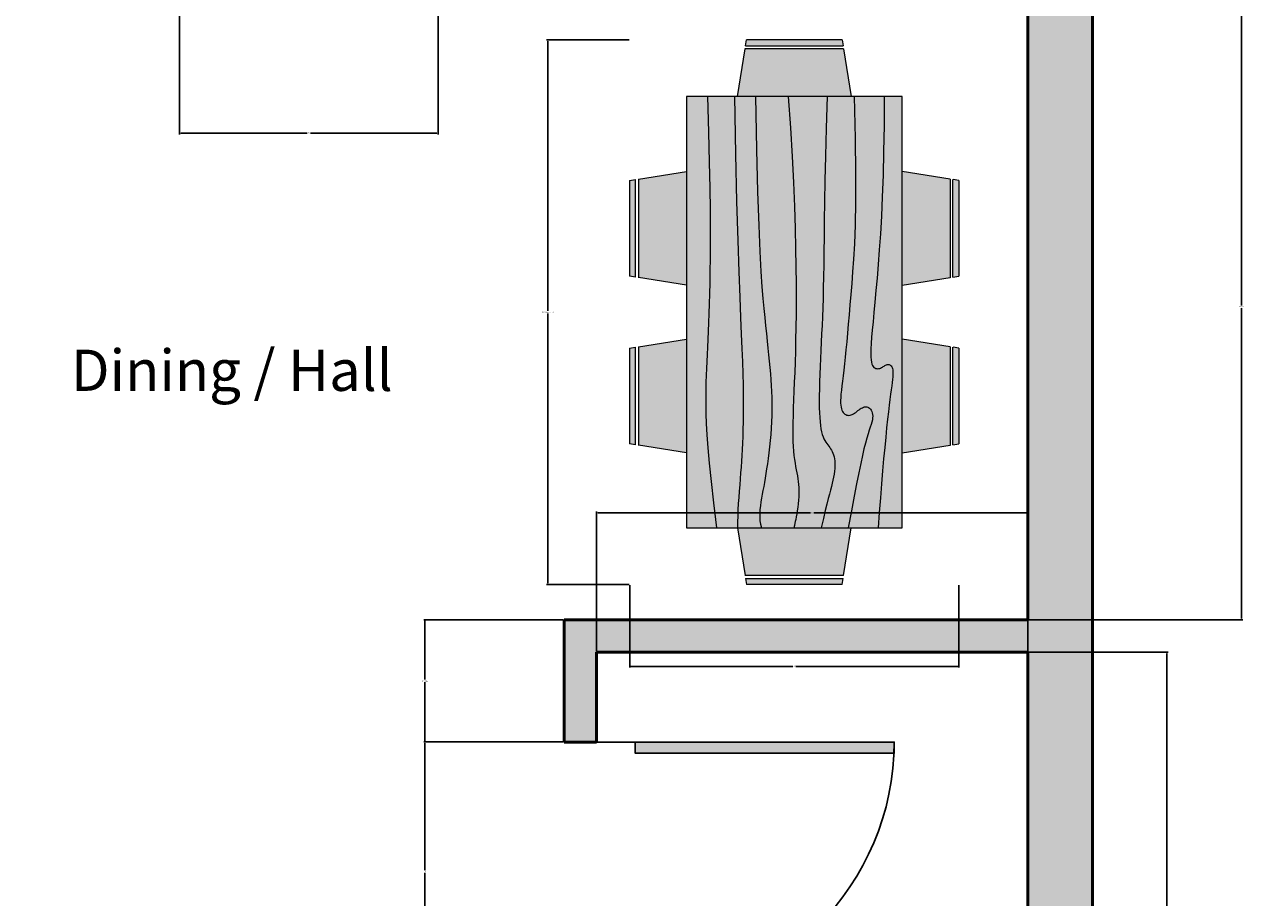
# Model space of a CAD drawing. Units: inches. Extents: x 2578 to 2919, y 51 to 451.
# Tile 4 of 5: x 2750 to 2919, y 172 to 293. Entities that reach past the tile are written whole.
import ezdxf

# ---------------------------------------------------------------- set-up
doc = ezdxf.new("R2010")
doc.units = ezdxf.units.IN
for name, color, linetype, lineweight in [('A-ANNO-DIMS', 2, 'Continuous', 18), ('A-AREA-IDEN', 7, 'Continuous', 25), ('A-DOOR', 4, 'Continuous', 25), ('A-FURN', 8, 'Continuous', 18), ('A-FURN-PATT', 253, 'Continuous', 13), ('A-WALL', 7, 'Continuous', 50), ('A-WALL-PATT', 250, 'Continuous', 13)]:
    doc.layers.add(name, color=color, linetype=linetype, lineweight=lineweight)
doc.layers.add('A-DOOR-PATT', color=29, linetype='Continuous', lineweight=13, true_color=0x4f342a)
doc.styles.get("Standard").update_dxf_attribs({"font": 'arial.ttf'})
doc.dimstyles.get("Standard").update_dxf_attribs({"dimtxt": 0.18, "dimasz": 0.18, "dimexe": 0.18, "dimexo": 0.0625, "dimgap": 0.09, "dimtad": 0, "dimtih": 1, "dimtoh": 1, "dimdec": 4, "dimzin": 0, "dimdsep": 46, "dimtxsty": 'Standard', "dimcen": 0.09, "dimadec": 0, "dimazin": 0, "dimtfac": 1, "dimtdec": 4, "dimtofl": 0, "dimtmove": 0, "dimatfit": 3, "dimfxl": 1, "dimtolj": 1, "dimtzin": 0, "dimarcsym": 0})

# ---------------------------------------------------------------- blocks, each defined once
blk = doc.blocks.new('*U3')
for p, q in [((0, 0), (0, -6)), ((40, 0), (40, -6))]:
    blk.add_line(p, q)
blk.add_lwpolyline([(0, 0), (0, 40), (1.75, 40), (1.75, 0)], close=True)
blk.add_arc((0, 0), 40, 0, 90)
blk = doc.blocks.new('Dining Set - 36 x 72 in.')
for p, q in [((-22, 27.5), (-22.1562, 26.50042)), ((-5.8416, 26.5), (-22.1534, 26.5)), ((-22, 27.5), (-6, 27.5)), ((-5.8437, 26.49966), (-6, 27.5)), ((6, 27.5), (5.8438, 26.50042)), ((22.1584, 26.5), (5.8466, 26.5)), ((6, 27.5), (22, 27.5)), ((22.1563, 26.49966), (22, 27.5)), ((-22.2343, 26.00059), (-23.4847, 17.99762)), ((-22.2304, 26), (-5.7608, 26)), ((-4.5152, 17.99762), (-5.7655, 25.99926)), ((5.7657, 26.00059), (4.5153, 17.99762)), ((5.7696, 26), (22.2392, 26)), ((23.4848, 17.99762), (22.2345, 25.99926)), ((36, 18), (-36, 18)), ((-36, 18), (-36, -18)), ((36, -18), (36, 18)), ((-45.5, 8), (-44.5004, 8.15617)), ((-44.5, -8.15843), (-44.5, 8.15338)), ((-44.0006, 8.23428), (-35.9976, 9.48474)), ((-44, 8.23041), (-44, -8.23915)), ((44.0006, 8.23428), (35.9976, 9.48474)), ((44, 8.23041), (44, -8.23915)), ((44.5, -8.15843), (44.5, 8.15338)), ((45.5, 8), (44.5005, 8.15617)), ((-45.5, 8), (-45.5, -8)), ((45.5, 8), (45.5, -8)), ((-44.4997, -8.15631), (-45.5, -8)), ((44.4997, -8.15631), (45.5, -8)), ((-35.9976, -9.48476), (-43.9993, -8.2345)), ((35.9976, -9.48476), (43.9993, -8.2345)), ((-36, -18), (36, -18)), ((-22.2343, -26.0006), (-23.4847, -17.99762)), ((-4.5152, -17.99762), (-5.7655, -25.99928)), ((5.7657, -26.0006), (4.5153, -17.99762)), ((23.4848, -17.99762), (22.2345, -25.99928)), ((-22.2304, -26), (-5.7608, -26)), ((5.7696, -26), (22.2392, -26)), ((-22, -27.5), (-22.1562, -26.50044)), ((-5.8416, -26.5), (-22.1534, -26.5)), ((-22, -27.5), (-6, -27.5)), ((-5.8437, -26.49967), (-6, -27.5)), ((6, -27.5), (5.8438, -26.50044)), ((22.1584, -26.5), (5.8466, -26.5)), ((6, -27.5), (22, -27.5)), ((22.1563, -26.49967), (22, -27.5))]:
    blk.add_line(p, q)
for points in [[(-36, 15), (-31.1772, 14.97754), (-26.8079, 14.91406), (-22.8538, 14.81543), (-19.276, 14.6875), (-16.0362, 14.53613), (-13.0957, 14.36718), (-10.4159, 14.18652), (-7.9583, 14), (-5.6904, 13.81315), (-3.6035, 13.63021), (-1.6954, 13.45508), (0.0365, 13.29166), (1.5945, 13.14388), (2.9811, 13.01562), (4.1988, 12.9108), (5.25, 12.83333), (6.1393, 12.78613), (6.8802, 12.76823), (7.4883, 12.77767), (7.9792, 12.8125), (8.3685, 12.87077), (8.6719, 12.95052), (8.9049, 13.0498), (9.0833, 13.16666), (9.2205, 13.29899), (9.3216, 13.44401), (9.3895, 13.59879), (9.4271, 13.76041), (9.4373, 13.92594), (9.4232, 14.09245), (9.3875, 14.257), (9.3333, 14.41666), (9.2638, 14.56917), (9.1836, 14.71484), (9.0975, 14.85465), (9.0104, 14.98958), (8.9272, 15.1206), (8.8529, 15.2487), (8.7922, 15.37483), (8.75, 15.5), (8.7305, 15.62467), (8.7344, 15.74739), (8.7617, 15.86621), (8.8125, 15.97916), (8.8867, 16.08431), (8.9844, 16.17968), (9.1055, 16.26334), (9.25, 16.33333), (9.4189, 16.38802), (9.6172, 16.42708), (9.8506, 16.45052), (10.125, 16.45833), (10.4463, 16.45052), (10.8203, 16.42708), (11.2529, 16.38802), (11.75, 16.33333), (12.3184, 16.26318), (12.9694, 16.17838), (13.7151, 16.07991), (14.5677, 15.96875), (15.5395, 15.84586), (16.6426, 15.71224), (17.8893, 15.56884), (19.2917, 15.41666), (20.859, 15.25667), (22.5879, 15.08984), (24.4721, 14.91715), (26.5052, 14.73958), (28.6809, 14.5581), (30.9929, 14.3737), (33.4347, 14.18733), (36, 14)], [(-36, 10), (-28.9766, 10.14274), (-23.1725, 10.20442), (-18.4241, 10.19775), (-14.5677, 10.13541), (-11.4399, 10.03011), (-8.877, 9.89453), (-6.7154, 9.74137), (-4.7917, 9.58333), (-2.9698, 9.43082), (-1.2246, 9.28515), (0.4415, 9.14534), (2.026, 9.01041), (3.5266, 8.87939), (4.9408, 8.7513), (6.266, 8.62516), (7.5, 8.5), (8.6411, 8.37549), (9.6914, 8.2539), (10.6538, 8.13818), (11.5312, 8.03125), (12.3267, 7.93603), (13.043, 7.85547), (13.6831, 7.79248), (14.25, 7.75), (14.7471, 7.7303), (15.1797, 7.73307), (15.5537, 7.75732), (15.875, 7.80208), (16.1494, 7.86637), (16.3828, 7.94922), (16.5811, 8.04964), (16.75, 8.16666), (16.8944, 8.29915), (17.0143, 8.44531), (17.1089, 8.60319), (17.1771, 8.77083), (17.218, 8.94629), (17.2305, 9.1276), (17.2137, 9.31282), (17.1667, 9.5), (17.0895, 9.6875), (16.987, 9.875), (16.8649, 10.0625), (16.7292, 10.25), (16.5856, 10.4375), (16.4401, 10.625), (16.2985, 10.8125), (16.1667, 11), (16.05, 11.18733), (15.9518, 11.3737), (15.8752, 11.5581), (15.8229, 11.73958), (15.798, 11.91715), (15.8034, 12.08984), (15.842, 12.25667), (15.9167, 12.41666), (16.0295, 12.56836), (16.1784, 12.70833), (16.3605, 12.83268), (16.5729, 12.9375), (16.8127, 13.01888), (17.0768, 13.07291), (17.3625, 13.0957), (17.6667, 13.08333), (17.9894, 13.03312), (18.3418, 12.94726), (18.7382, 12.82918), (19.1927, 12.68229), (19.7195, 12.51001), (20.3327, 12.31575), (21.0465, 12.10294), (21.875, 11.875), (22.8357, 11.63354), (23.959, 11.37304), (25.2786, 11.08618), (26.8282, 10.76562), (28.6414, 10.40405), (30.752, 9.99414), (33.1936, 9.52856), (36, 9)], [(-36, 5.5), (-30.7157, 5.3348), (-26.069, 5.20963), (-21.9946, 5.11767), (-18.4271, 5.05208), (-15.3009, 5.00602), (-12.5508, 4.97265), (-10.1112, 4.94515), (-7.9167, 4.91666), (-5.909, 4.88167), (-4.0586, 4.83984), (-2.3429, 4.79215), (-0.7396, 4.73958), (0.7739, 4.6831), (2.22, 4.6237), (3.6213, 4.56233), (5, 4.5), (6.373, 4.43782), (7.7344, 4.3776), (9.0723, 4.32129), (10.375, 4.27083), (11.6309, 4.22819), (12.8281, 4.19531), (13.9551, 4.17415), (15, 4.16666), (15.954, 4.17448), (16.819, 4.19791), (17.6001, 4.23698), (18.3021, 4.29166), (18.9299, 4.36198), (19.4883, 4.44791), (19.9823, 4.54948), (20.4167, 4.66666), (20.7969, 4.79899), (21.1302, 4.94401), (21.4245, 5.09879), (21.6875, 5.26041), (21.9271, 5.42594), (22.1511, 5.59245), (22.3672, 5.757), (22.5834, 5.91666), (22.8065, 6.06868), (23.0404, 6.21093), (23.2879, 6.34147), (23.5521, 6.45833), (23.8358, 6.55957), (24.142, 6.64323), (24.4735, 6.70735), (24.8334, 6.75), (25.2235, 6.76969), (25.642, 6.76692), (26.0858, 6.74267), (26.5521, 6.69791), (27.0379, 6.63362), (27.5404, 6.55078), (28.0565, 6.45036), (28.5834, 6.33333), (29.1242, 6.19987), (29.7071, 6.04687), (30.3661, 5.87044), (31.1354, 5.66666), (32.0493, 5.43164), (33.142, 5.16146), (34.4475, 4.85221), (36, 4.5)], [(-36, -1), (-30.7915, -0.6591), (-26.0195, -0.38216), (-21.6519, -0.16284), (-17.6563, 0.00521), (-14.0005, 0.12833), (-10.6523, 0.21289), (-7.5796, 0.26522), (-4.75, 0.29166), (-2.134, 0.29793), (0.2878, 0.28711), (2.5317, 0.26163), (4.6146, 0.22396), (6.5529, 0.17651), (8.3633, 0.12174), (10.0623, 0.06209), (11.6667, 0), (13.1899, -0.06201), (14.6341, -0.1211), (15.9982, -0.17432), (17.2813, -0.21875), (18.4823, -0.25147), (19.6003, -0.26953), (20.6343, -0.27002), (21.5834, -0.25), (22.4481, -0.20768), (23.2357, -0.14584), (23.9549, -0.06836), (24.6146, 0.02083), (25.2235, 0.11784), (25.7904, 0.21875), (26.3241, 0.31966), (26.8334, 0.41666), (27.3265, 0.50618), (27.8099, 0.58593), (28.2894, 0.65397), (28.7709, 0.70833), (29.2601, 0.74707), (29.763, 0.76823), (30.2855, 0.76985), (30.8334, 0.75), (31.4088, 0.70784), (31.9994, 0.64713), (32.589, 0.57275), (33.1615, 0.48958), (33.7008, 0.4025), (34.1908, 0.3164), (34.6153, 0.23616), (34.9584, 0.16666), (35.2099, 0.11165), (35.3848, 0.07031), (35.504, 0.04069), (35.5886, 0.02083), (35.6594, 0.00879), (35.7377, 0.0026), (35.8442, 0.00032), (36, 0)], [(-36, -6.5), (-27.1843, -6.31267), (-20.084, -6.1263), (-14.469, -5.9419), (-10.1094, -5.76042), (-6.7752, -5.58285), (-4.2363, -5.41016), (-2.2629, -5.24333), (-0.625, -5.08334), (0.8708, -4.93099), (2.2715, -4.78646), (3.5872, -4.64974), (4.8281, -4.52084), (6.0046, -4.39974), (7.127, -4.28646), (8.2053, -4.18099), (9.25, -4.08334), (10.2705, -3.99382), (11.2734, -3.91407), (12.2647, -3.84603), (13.25, -3.79167), (14.2354, -3.75293), (15.2266, -3.73177), (16.2295, -3.73015), (17.25, -3.75), (18.2912, -3.79248), (19.3451, -3.85547), (20.4009, -3.93604), (21.4479, -4.03125), (22.4754, -4.13819), (23.4727, -4.25391), (24.4289, -4.37549), (25.3334, -4.5), (26.1785, -4.62492), (26.9694, -4.74935), (27.7145, -4.87281), (28.4219, -4.99479), (29.1, -5.11483), (29.7572, -5.23242), (30.4016, -5.34709), (31.0417, -5.45834), (31.6837, -5.56437), (32.3262, -5.65821), (32.9658, -5.73153), (33.599, -5.77604), (34.2224, -5.78345), (34.8327, -5.74545), (35.4264, -5.65373), (36, -5.5)], [(-36, -10), (-26.4022, -9.81299), (-18.4675, -9.62891), (-11.9839, -9.45069), (-6.7396, -9.28125), (-2.5226, -9.12354), (0.8789, -8.98047), (3.6769, -8.85498), (6.0833, -8.75), (8.2767, -8.66765), (10.3021, -8.60677), (12.1712, -8.56543), (13.8958, -8.54167), (15.4876, -8.53353), (16.9583, -8.53907), (18.3197, -8.55632), (19.5834, -8.58334), (20.7616, -8.61841), (21.8685, -8.66081), (22.9188, -8.71004), (23.9271, -8.76563), (24.9081, -8.82707), (25.8763, -8.89388), (26.8465, -8.96558), (27.8334, -9.04167), (28.8474, -9.12118), (29.8828, -9.20117), (30.93, -9.27824), (31.9792, -9.34896), (33.0205, -9.40991), (34.0443, -9.45768), (35.0407, -9.48885), (36, -9.5)], [(-36, -14.5), (-30.0881, -14.33513), (-25.0332, -14.21224), (-20.7312, -14.12647), (-17.0781, -14.07292), (-13.97, -14.04671), (-11.3027, -14.04297), (-8.9724, -14.05681), (-6.875, -14.08334), (-4.9224, -14.11833), (-3.0905, -14.16016), (-1.3709, -14.20785), (0.2448, -14.26042), (1.7647, -14.3169), (3.1973, -14.3763), (4.5507, -14.43767), (5.8333, -14.5), (7.0554, -14.5621), (8.235, -14.62175), (9.3922, -14.67652), (10.5469, -14.72396), (11.7192, -14.76164), (12.929, -14.78711), (14.1965, -14.79794), (15.5417, -14.79167), (16.9933, -14.76424), (18.6152, -14.70508), (20.4804, -14.60197), (22.6615, -14.44271), (25.2312, -14.21509), (28.2624, -13.9069), (31.8277, -13.50594), (36, -13)]]:
    blk.add_lwpolyline(points)
blk = doc.blocks.new('*D27')
at = {"layer": 'A-ANNO-DIMS', "color": 0, "lineweight": -2, "transparency": 16777216}
for p, q in [((2833.73, 291.27), (2822.25, 291.27)), ((2822.43, 291.09), (2822.43, 253.56)), ((2822.43, 215.67), (2822.43, 253.2)), ((2833.73, 215.49), (2822.25, 215.49))]:
    blk.add_line(p, q, dxfattribs=at)
at = {"layer": 'A-ANNO-DIMS', "color": 0, "transparency": 16777216}
for points in [[(2822.4, 291.09), (2822.46, 291.09), (2822.43, 291.27)], [(2822.4, 215.67), (2822.46, 215.67), (2822.43, 215.49)]]:
    blk.add_solid(points, dxfattribs=at)
at = {"layer": 'Defpoints', "color": 0, "transparency": 16777216}
for p in [(2833.8, 291.27), (2822.43, 215.49), (2833.8, 215.49)]:
    blk.add_point(p, dxfattribs=at)
at = {"layer": 'A-ANNO-DIMS', "color": 0, "transparency": 16777216, "insert": (2822.43, 253.38), "char_height": 0.18, "attachment_point": 5}
blk.add_mtext('\\A1;DINING SET 76', dxfattribs=at)
blk = doc.blocks.new('*D28')
at = {"layer": 'A-ANNO-DIMS', "color": 0, "lineweight": -2, "transparency": 16777216}
for p, q in [((2833.8, 215.43), (2833.8, 203.94)), ((2879.6, 215.43), (2879.6, 203.94)), ((2833.98, 204.12), (2856.48, 204.12)), ((2879.42, 204.12), (2856.92, 204.12))]:
    blk.add_line(p, q, dxfattribs=at)
at = {"layer": 'A-ANNO-DIMS', "color": 0, "transparency": 16777216}
for points in [[(2833.98, 204.15), (2833.98, 204.09), (2833.8, 204.12)], [(2879.42, 204.15), (2879.42, 204.09), (2879.6, 204.12)]]:
    blk.add_solid(points, dxfattribs=at)
at = {"layer": 'Defpoints', "color": 0, "transparency": 16777216}
for p in [(2833.8, 215.49), (2879.6, 215.49), (2879.6, 204.12)]:
    blk.add_point(p, dxfattribs=at)
at = {"layer": 'A-ANNO-DIMS', "color": 0, "transparency": 16777216, "insert": (2856.7, 204.12), "char_height": 0.18, "attachment_point": 5}
blk.add_mtext('\\A1;46', dxfattribs=at)
blk = doc.blocks.new('*D46')
at = {"layer": 'A-ANNO-DIMS', "color": 0, "lineweight": -2, "transparency": 16777216}
for p, q in [((2829.18, 206.17), (2829.18, 225.64)), ((2889.18, 206.17), (2889.18, 225.64)), ((2829.36, 225.46), (2858.96, 225.46)), ((2889, 225.46), (2859.4, 225.46))]:
    blk.add_line(p, q, dxfattribs=at)
at = {"layer": 'A-ANNO-DIMS', "color": 0, "transparency": 16777216}
for points in [[(2829.36, 225.49), (2829.36, 225.43), (2829.18, 225.46)], [(2889, 225.49), (2889, 225.43), (2889.18, 225.46)]]:
    blk.add_solid(points, dxfattribs=at)
at = {"layer": 'Defpoints', "color": 0, "transparency": 16777216}
for p in [(2889.18, 225.46), (2829.18, 206.11), (2889.18, 206.11)]:
    blk.add_point(p, dxfattribs=at)
at = {"layer": 'A-ANNO-DIMS', "color": 0, "transparency": 16777216, "insert": (2859.18, 225.46), "char_height": 0.18, "attachment_point": 5}
blk.add_mtext('\\A1;60', dxfattribs=at)
blk = doc.blocks.new('*D47')
at = {"layer": 'A-ANNO-DIMS', "color": 0, "lineweight": -2, "transparency": 16777216}
for p, q in [((2889.24, 206.11), (2908.71, 206.11)), ((2908.53, 205.93), (2908.53, 153.04)), ((2908.53, 99.78), (2908.53, 152.67)), ((2889.24, 99.6), (2908.71, 99.6))]:
    blk.add_line(p, q, dxfattribs=at)
at = {"layer": 'A-ANNO-DIMS', "color": 0, "transparency": 16777216}
for points in [[(2908.5, 205.93), (2908.56, 205.93), (2908.53, 206.11)], [(2908.5, 99.78), (2908.56, 99.78), (2908.53, 99.6)]]:
    blk.add_solid(points, dxfattribs=at)
at = {"layer": 'Defpoints', "color": 0, "transparency": 16777216}
for p in [(2889.18, 206.11), (2889.18, 99.6), (2908.53, 99.6)]:
    blk.add_point(p, dxfattribs=at)
at = {"layer": 'A-ANNO-DIMS', "color": 0, "transparency": 16777216, "insert": (2908.53, 152.85), "char_height": 0.18, "attachment_point": 5}
blk.add_mtext('\\A1;106.51', dxfattribs=at)
blk = doc.blocks.new('*D49')
at = {"layer": 'A-ANNO-DIMS', "color": 0, "lineweight": -2, "transparency": 16777216}
for p, q in [((2889.24, 297.64), (2919.06, 297.64)), ((2918.88, 297.46), (2918.88, 254.31)), ((2918.88, 210.79), (2918.88, 253.94)), ((2889.24, 210.61), (2919.06, 210.61))]:
    blk.add_line(p, q, dxfattribs=at)
at = {"layer": 'A-ANNO-DIMS', "color": 0, "transparency": 16777216}
for points in [[(2918.85, 297.46), (2918.91, 297.46), (2918.88, 297.64)], [(2918.85, 210.79), (2918.91, 210.79), (2918.88, 210.61)]]:
    blk.add_solid(points, dxfattribs=at)
at = {"layer": 'Defpoints', "color": 0, "transparency": 16777216}
for p in [(2889.18, 297.64), (2918.88, 297.64), (2889.18, 210.61)]:
    blk.add_point(p, dxfattribs=at)
at = {"layer": 'A-ANNO-DIMS', "color": 0, "transparency": 16777216, "insert": (2918.88, 254.13), "char_height": 0.18, "attachment_point": 5}
blk.add_mtext('\\A1;87.03', dxfattribs=at)
blk = doc.blocks.new('*D54')
at = {"layer": 'A-ANNO-DIMS', "color": 0, "lineweight": -2, "transparency": 16777216}
for p, q in [((2771.18, 297.58), (2771.18, 278.11)), ((2807.18, 297.58), (2807.18, 278.11)), ((2771.36, 278.29), (2788.96, 278.29)), ((2807, 278.29), (2789.4, 278.29))]:
    blk.add_line(p, q, dxfattribs=at)
at = {"layer": 'A-ANNO-DIMS', "color": 0, "transparency": 16777216}
for points in [[(2771.36, 278.32), (2771.36, 278.26), (2771.18, 278.29)], [(2807, 278.32), (2807, 278.26), (2807.18, 278.29)]]:
    blk.add_solid(points, dxfattribs=at)
at = {"layer": 'Defpoints', "color": 0, "transparency": 16777216}
for p in [(2771.18, 297.64), (2807.18, 297.64), (2771.18, 278.29)]:
    blk.add_point(p, dxfattribs=at)
at = {"layer": 'A-ANNO-DIMS', "color": 0, "transparency": 16777216, "insert": (2789.18, 278.29), "char_height": 0.18, "attachment_point": 5}
blk.add_mtext('\\A1;36', dxfattribs=at)
blk = doc.blocks.new('*D57')
at = {"layer": 'A-ANNO-DIMS', "color": 0, "lineweight": -2, "transparency": 16777216}
for p, q in [((2824.62, 193.6), (2805.15, 193.6)), ((2805.33, 193.42), (2805.33, 175.78)), ((2805.33, 157.78), (2805.33, 175.42)), ((2824.62, 157.6), (2805.15, 157.6))]:
    blk.add_line(p, q, dxfattribs=at)
at = {"layer": 'A-ANNO-DIMS', "color": 0, "transparency": 16777216}
for points in [[(2805.3, 193.42), (2805.36, 193.42), (2805.33, 193.6)], [(2805.3, 157.78), (2805.36, 157.78), (2805.33, 157.6)]]:
    blk.add_solid(points, dxfattribs=at)
at = {"layer": 'Defpoints', "color": 0, "transparency": 16777216}
for p in [(2805.33, 193.6), (2824.68, 193.6), (2824.68, 157.6)]:
    blk.add_point(p, dxfattribs=at)
at = {"layer": 'A-ANNO-DIMS', "color": 0, "transparency": 16777216, "insert": (2805.33, 175.6), "char_height": 0.18, "attachment_point": 5}
blk.add_mtext('\\A1;36', dxfattribs=at)
blk = doc.blocks.new('*D58')
at = {"layer": 'A-ANNO-DIMS', "color": 0, "lineweight": -2, "transparency": 16777216}
for p, q in [((2824.62, 210.61), (2805.15, 210.61)), ((2805.33, 210.43), (2805.33, 202.29)), ((2805.33, 193.78), (2805.33, 201.92)), ((2824.62, 193.6), (2805.15, 193.6))]:
    blk.add_line(p, q, dxfattribs=at)
at = {"layer": 'A-ANNO-DIMS', "color": 0, "transparency": 16777216}
for points in [[(2805.3, 210.43), (2805.36, 210.43), (2805.33, 210.61)], [(2805.3, 193.78), (2805.36, 193.78), (2805.33, 193.6)]]:
    blk.add_solid(points, dxfattribs=at)
at = {"layer": 'Defpoints', "color": 0, "transparency": 16777216}
for p in [(2805.33, 210.61), (2824.68, 210.61), (2824.68, 193.6)]:
    blk.add_point(p, dxfattribs=at)
at = {"layer": 'A-ANNO-DIMS', "color": 0, "transparency": 16777216, "insert": (2805.33, 202.1), "char_height": 0.18, "attachment_point": 5}
blk.add_mtext('\\A1;17.012', dxfattribs=at)

msp = doc.modelspace()

# ---------------------------------------------------------------- hatches: boundary and pattern name
at = {"layer": 'A-DOOR-PATT'}
h = msp.add_hatch(color=256, dxfattribs=at)
h.dxf.hatch_style = 1
h.paths.add_polyline_path([(2717.5545, 331.5492, 0.01094143), (2715.9791, 331.5147), (2715.9791, 295.5417), (2717.5545, 295.5417)])
h.paths.add_polyline_path([(2772.7563, 343.5147, 0.01094143), (2771.181, 343.5492), (2771.181, 307.5417), (2772.7563, 307.5417)])
h.paths.add_polyline_path([(2809.181, 302.1406), (2807.181, 302.1406), (2807.181, 297.6406), (2809.181, 297.6406)])
h.paths.add_polyline_path([(2681.547, 290.1406), (2679.547, 290.1406), (2679.547, 285.6406), (2681.547, 285.6406)])
h.paths.add_polyline_path([(2870.5896, 193.5988), (2834.5821, 193.5988), (2834.5821, 192.0235), (2870.5551, 192.0235, 0.01094143)])
h.paths.add_polyline_path([(2829.181, 157.5988), (2824.681, 157.5988), (2824.681, 155.5988), (2829.181, 155.5988)])
h.paths.add_polyline_path([(2702.547, 145.6406), (2698.047, 145.6406), (2698.047, 143.6481), (2702.547, 143.6481)])
h.paths.add_polyline_path([(2697.1459, 109.2159), (2661.1384, 109.2159), (2661.1384, 107.6406), (2697.1459, 107.6406)])
h.paths.add_polyline_path([(2702.547, 107.6406), (2698.047, 107.6406), (2698.047, 105.6406), (2702.547, 105.6406)])
h.paths.add_polyline_path([(2771.181, 302.1406), (2769.181, 302.1406), (2769.181, 297.6406), (2771.181, 297.6406)])
at = {"layer": 'A-FURN-PATT'}
h = msp.add_hatch(color=256, dxfattribs=at)
h.dxf.hatch_style = 1
h.paths.add_polyline_path([(2668.0284, 410.6078), (2629.3175, 410.6078), (2629.3175, 398.9331), (2619.4862, 398.9331), (2619.4862, 364.5234), (2668.0284, 364.5234)])
h.paths.add_polyline_path([(2617.6428, 398.9331), (2619.1789, 400.4692), (2619.1789, 404.4632), (2607.5042, 404.4632), (2607.5042, 388.4873), (2617.6428, 388.4873)])
h.paths.add_polyline_path([(2617.6428, 386.6439), (2607.5042, 386.6439), (2607.5042, 370.668), (2617.6428, 370.668)])
h.paths.add_polyline_path([(2875.6753, 403.5558), (2825.7487, 403.5558), (2825.7487, 356.1571), (2865.5636, 356.1571), (2865.5636, 368.1648), (2875.6753, 368.1648)])
h.paths.add_polyline_path([(2887.999, 397.2359), (2877.5713, 397.2359), (2877.5713, 380.8044), (2887.999, 380.8044)])
h.paths.add_polyline_path([(2887.999, 378.9085), (2877.5713, 378.9085), (2877.5713, 368.1648), (2875.9913, 366.5848), (2875.9913, 362.4769), (2887.999, 362.4769)])
h.paths.add_polyline_path([(2863.3609, 291.2749), (2850.0358, 291.2749), (2849.9056, 290.442), (2863.4911, 290.442)])
h.paths.add_polyline_path([(2834.6285, 271.8336), (2833.7957, 271.7035), (2833.7957, 258.3783), (2834.6285, 258.2482)])
h.paths.add_polyline_path([(2834.6285, 248.5146), (2833.7957, 248.3844), (2833.7957, 235.0593), (2834.6285, 234.9291)])
h.paths.add_polyline_path([(2879.601, 248.3844), (2878.7682, 248.5146), (2878.7682, 234.9291), (2879.601, 235.0593)])
h.paths.add_polyline_path([(2879.601, 271.7035), (2878.7682, 271.8336), (2878.7682, 258.2482), (2879.601, 258.3783)])
h.paths.add_polyline_path([(2863.4911, 216.3207), (2849.9056, 216.3207), (2850.0358, 215.4879), (2863.3609, 215.4879)])
h.paths.add_polyline_path([(2875.3365, 114.2473, 0.48007965), (2857.7894, 112.0785, 0.21500378), (2857.7543, 108.7906, 0.4800795), (2875.2511, 106.2478)])
h.paths.add_polyline_path([(2880.9002, 120.1884), (2879.9002, 120.199), (2879.8682, 117.1992), (2881.3682, 117.1832), (2881.3788, 118.1831), (2880.8789, 118.1885)])
h.paths.add_polyline_path([(2888.3838, 118.6084, 0.50000012), (2887.3945, 119.619), (2883.3947, 119.6617, 0.50000012), (2882.3841, 118.6724), (2882.2027, 101.6734, 0.50000012), (2883.192, 100.6628), (2887.1918, 100.6201, 0.50000012), (2888.2024, 101.6094)])
h = msp.add_hatch(color=256, dxfattribs=at)
h.dxf.hatch_style = 1
h.paths.add_polyline_path([(2841.7075, 272.9397), (2835.0449, 271.8987), (2835.0449, 258.1831), (2841.7075, 257.1421)])
h.paths.add_polyline_path([(2841.7075, 249.6206), (2835.0449, 248.5797), (2835.0449, 234.8641), (2841.7075, 233.823)])
h.paths.add_polyline_path([(2878.3518, 248.5797), (2871.6892, 249.6206), (2871.6892, 233.823), (2878.3518, 234.8641)])
h.paths.add_polyline_path([(2878.3518, 271.8987), (2871.6892, 272.9397), (2871.6892, 257.1421), (2878.3518, 258.1831)])
h.paths.add_polyline_path([(2863.5561, 290.0256), (2849.8406, 290.0256), (2848.7995, 283.363), (2864.5972, 283.363)])
h.paths.add_polyline_path([(2864.5972, 223.3997), (2848.7995, 223.3997), (2849.8406, 216.7371), (2863.5561, 216.7371)])
h = msp.add_hatch(color=256, dxfattribs=at)
h.dxf.hatch_style = 1
h.paths.add_polyline_path([(2844.9403, 257.4809), (2844.9694, 259.107), (2844.9915, 260.8538), (2845.003, 262.7945), (2844.9999, 265.0159), (2844.9781, 267.6044), (2844.9335, 270.6468), (2844.8621, 274.2296), (2844.7597, 278.4395), (2844.6224, 283.363), (2841.7075, 283.363), (2841.7075, 223.3997), (2845.8717, 223.3997), (2845.4503, 226.8745), (2845.1164, 229.8438), (2844.8597, 232.3682), (2844.6701, 234.5084), (2844.5375, 236.3248), (2844.4516, 237.8782), (2844.4024, 239.229), (2844.3795, 240.4379), (2844.3743, 241.5582), (2844.3833, 242.6138), (2844.4045, 243.6214), (2844.4359, 244.5977), (2844.4754, 245.5593), (2844.521, 246.5231), (2844.5707, 247.5055), (2844.6224, 248.5233), (2844.6743, 249.5915), (2844.7254, 250.7186), (2844.7749, 251.9117), (2844.8219, 253.1775), (2844.8657, 254.5231), (2844.9054, 255.9552)])
h.paths.add_polyline_path([(2849.4112, 248.3151), (2849.3237, 250.3192), (2849.2192, 252.6494), (2849.1001, 255.4823), (2848.9687, 258.9943), (2848.8276, 263.3619), (2848.6792, 268.7616), (2848.5259, 275.3698), (2848.3701, 283.363), (2844.6224, 283.363), (2844.7597, 278.4395), (2844.8621, 274.2296), (2844.9335, 270.6468), (2844.9781, 267.6044), (2844.9999, 265.0159), (2845.003, 262.7945), (2844.9915, 260.8538), (2844.9694, 259.107), (2844.9403, 257.4809), (2844.9054, 255.9552), (2844.8657, 254.5231), (2844.8219, 253.1775), (2844.7749, 251.9117), (2844.7254, 250.7186), (2844.6743, 249.5915), (2844.6224, 248.5233), (2844.5707, 247.5055), (2844.521, 246.5231), (2844.4754, 245.5593), (2844.4359, 244.5977), (2844.4045, 243.6214), (2844.3833, 242.6138), (2844.3743, 241.5582), (2844.3795, 240.4379), (2844.4024, 239.229), (2844.4516, 237.8782), (2844.5375, 236.3248), (2844.6701, 234.5084), (2844.8597, 232.3682), (2845.1164, 229.8438), (2845.4503, 226.8745), (2845.8717, 223.3997), (2848.7865, 223.3997), (2848.7958, 224.1987), (2848.8218, 225.0285), (2848.8616, 225.8811), (2848.9123, 226.7484), (2848.9712, 227.6222), (2849.0354, 228.4943), (2849.102, 229.3566), (2849.1682, 230.2011), (2849.2316, 231.023), (2849.2913, 231.831), (2849.347, 232.6373), (2849.3981, 233.4543), (2849.4444, 234.2941), (2849.4854, 235.1688), (2849.5207, 236.0906), (2849.55, 237.0719), (2849.5725, 238.1243), (2849.5868, 239.2581), (2849.5914, 240.4829), (2849.5847, 241.8086), (2849.5649, 243.2449), (2849.5304, 244.8016), (2849.4797, 246.4884)])
h.paths.add_polyline_path([(2853.5728, 241.5258), (2853.5406, 242.3465), (2853.4953, 243.1671), (2853.4386, 243.9926), (2853.3722, 244.8279), (2853.2977, 245.6778), (2853.2163, 246.5478), (2853.1285, 247.4459), (2853.0342, 248.3806), (2852.9333, 249.3604), (2852.8259, 250.3939), (2852.7121, 251.4896), (2852.5917, 252.6562), (2852.4648, 253.9019), (2852.3316, 255.266), (2852.1927, 256.9095), (2852.0488, 259.0239), (2851.9009, 261.8007), (2851.7498, 265.4315), (2851.5962, 270.1078), (2851.441, 276.0211), (2851.285, 283.363), (2848.3701, 283.363), (2848.5259, 275.3698), (2848.6792, 268.7616), (2848.8276, 263.3619), (2848.9687, 258.9943), (2849.1001, 255.4823), (2849.2192, 252.6494), (2849.3237, 250.3192), (2849.4112, 248.3151), (2849.4797, 246.4884), (2849.5304, 244.8016), (2849.5649, 243.2449), (2849.5847, 241.8086), (2849.5914, 240.4829), (2849.5868, 239.2581), (2849.5725, 238.1243), (2849.55, 237.0719), (2849.5207, 236.0906), (2849.4854, 235.1688), (2849.4444, 234.2941), (2849.3981, 233.4543), (2849.347, 232.6373), (2849.2913, 231.831), (2849.2316, 231.023), (2849.1682, 230.2011), (2849.102, 229.3566), (2849.0354, 228.4943), (2848.9712, 227.6222), (2848.9123, 226.7484), (2848.8616, 225.8811), (2848.8218, 225.0285), (2848.7958, 224.1987), (2848.7874, 223.4772), (2848.7995, 223.3997), (2852.1178, 223.3997), (2851.9898, 223.8774), (2851.9134, 224.3719), (2851.8818, 224.8802), (2851.8879, 225.3993), (2851.925, 225.9267), (2851.9861, 226.4594), (2852.0642, 226.9945), (2852.1525, 227.5291), (2852.2452, 228.0622), (2852.3407, 228.5989), (2852.4386, 229.1462), (2852.5386, 229.711), (2852.6402, 230.3001), (2852.743, 230.9206), (2852.8466, 231.5793), (2852.9507, 232.2831), (2853.0543, 233.0364), (2853.1556, 233.8328), (2853.252, 234.6633), (2853.341, 235.5191), (2853.4203, 236.391), (2853.4874, 237.2703), (2853.5399, 238.148), (2853.5753, 239.0152), (2853.5918, 239.8651), (2853.5905, 240.7003)])
h.paths.add_polyline_path([(2856.5254, 234.6861), (2856.4902, 235.4062), (2856.4735, 236.1967), (2856.4739, 237.0578), (2856.4889, 237.9889), (2856.5162, 238.9891), (2856.5532, 240.0577), (2856.5975, 241.1938), (2856.6467, 242.3965), (2856.6984, 243.6651), (2856.7501, 245.0013), (2856.7997, 246.4162), (2856.8454, 247.924), (2856.8849, 249.5382), (2856.9163, 251.2729), (2856.9375, 253.1417), (2856.9465, 255.1586), (2856.9413, 257.3373), (2856.9192, 259.6939), (2856.8757, 262.2529), (2856.8052, 265.0413), (2856.7027, 268.086), (2856.5627, 271.4136), (2856.3801, 275.051), (2856.1494, 279.0253), (2855.8655, 283.363), (2851.285, 283.363), (2851.441, 276.0211), (2851.5962, 270.1078), (2851.7498, 265.4315), (2851.9009, 261.8007), (2852.0488, 259.0239), (2852.1927, 256.9095), (2852.3316, 255.266), (2852.4648, 253.9019), (2852.5917, 252.6562), (2852.7121, 251.4896), (2852.8259, 250.3939), (2852.9333, 249.3604), (2853.0342, 248.3806), (2853.1285, 247.4459), (2853.2163, 246.5478), (2853.2977, 245.6778), (2853.3722, 244.8279), (2853.4386, 243.9926), (2853.4953, 243.1671), (2853.5406, 242.3465), (2853.5728, 241.5258), (2853.5905, 240.7003), (2853.5918, 239.8651), (2853.5753, 239.0152), (2853.5399, 238.148), (2853.4874, 237.2703), (2853.4203, 236.391), (2853.341, 235.5191), (2853.252, 234.6633), (2853.1556, 233.8328), (2853.0543, 233.0364), (2852.9507, 232.2831), (2852.8466, 231.5793), (2852.743, 230.9206), (2852.6402, 230.3001), (2852.5386, 229.711), (2852.4386, 229.1462), (2852.3407, 228.5989), (2852.2452, 228.0622), (2852.1525, 227.5291), (2852.0642, 226.9945), (2851.9861, 226.4594), (2851.925, 225.9267), (2851.8879, 225.3993), (2851.8818, 224.8802), (2851.9134, 224.3719), (2851.9898, 223.8774), (2852.1178, 223.3997), (2856.6984, 223.3997), (2856.6989, 223.6708), (2856.7322, 223.8128), (2856.7569, 223.9121), (2856.7913, 224.0578), (2856.8372, 224.2672), (2856.895, 224.5529), (2856.9619, 224.9065), (2857.0336, 225.3146), (2857.1061, 225.7637), (2857.1754, 226.2405), (2857.2373, 226.7315), (2857.2879, 227.2234), (2857.323, 227.7026), (2857.3395, 228.1589), (2857.3382, 228.5941), (2857.3205, 229.0129), (2857.2883, 229.4203), (2857.243, 229.8213), (2857.1863, 230.2206), (2857.1199, 230.6232), (2857.0454, 231.0339), (2856.9646, 231.4581), (2856.8805, 231.9025), (2856.7965, 232.3747), (2856.7157, 232.8818), (2856.6414, 233.4312), (2856.5769, 234.0301)])
h.paths.add_polyline_path([(2862.3363, 232.3747), (2862.3199, 232.6995), (2862.2844, 232.9993), (2862.231, 233.2754), (2862.1613, 233.5304), (2862.077, 233.7666), (2861.9797, 233.9867), (2861.871, 234.1928), (2861.7525, 234.3876), (2861.6259, 234.5734), (2861.4929, 234.7535), (2861.2503, 235.0721), (2861.0794, 235.3195), (2860.9448, 235.5386), (2860.8158, 235.7837), (2860.6951, 236.0612), (2860.5849, 236.3779), (2860.4873, 236.7397), (2860.4027, 237.1511), (2860.3311, 237.6161), (2860.2726, 238.139), (2860.227, 238.7236), (2860.1945, 239.3741), (2860.175, 240.0945), (2860.1685, 240.889), (2860.1747, 241.7593), (2860.1923, 242.6978), (2860.2197, 243.6949), (2860.2552, 244.7408), (2860.2972, 245.8258), (2860.3441, 246.94), (2860.3943, 248.0738), (2860.4461, 249.2173), (2860.498, 250.3655), (2860.5491, 251.5325), (2860.5986, 252.7369), (2860.6456, 253.9973), (2860.6894, 255.3326), (2860.7291, 256.7615), (2860.7639, 258.3025), (2860.7931, 259.9746), (2860.8168, 261.8022), (2860.8397, 263.834), (2860.8675, 266.1243), (2860.9059, 268.7279), (2860.9605, 271.699), (2861.0371, 275.0923), (2861.1413, 278.9621), (2861.2789, 283.363), (2855.8655, 283.363), (2856.1494, 279.0253), (2856.3801, 275.051), (2856.5627, 271.4136), (2856.7027, 268.086), (2856.8052, 265.0413), (2856.8757, 262.2529), (2856.9192, 259.6939), (2856.9413, 257.3373), (2856.9465, 255.1586), (2856.9375, 253.1417), (2856.9163, 251.2729), (2856.8849, 249.5382), (2856.8454, 247.924), (2856.7997, 246.4162), (2856.7501, 245.0013), (2856.6984, 243.6651), (2856.6467, 242.3965), (2856.5975, 241.1938), (2856.5532, 240.0577), (2856.5162, 238.9891), (2856.4889, 237.9889), (2856.4739, 237.0578), (2856.4735, 236.1967), (2856.4902, 235.4062), (2856.5254, 234.6861), (2856.5769, 234.0301), (2856.6414, 233.4312), (2856.7157, 232.8818), (2856.7965, 232.3747), (2856.8805, 231.9025), (2856.9646, 231.4581), (2857.0454, 231.0339), (2857.1199, 230.6232), (2857.1863, 230.2206), (2857.243, 229.8213), (2857.2883, 229.4203), (2857.3205, 229.0129), (2857.3382, 228.5941), (2857.3395, 228.1589), (2857.323, 227.7026), (2857.2879, 227.2234), (2857.2373, 226.7315), (2857.1754, 226.2405), (2857.1061, 225.7637), (2857.0336, 225.3146), (2856.9619, 224.9065), (2856.895, 224.5529), (2856.815, 224.1579), (2856.7129, 223.7259), (2856.7057, 223.6834), (2856.7005, 223.6182), (2856.6986, 223.5295), (2856.6984, 223.3997), (2860.4461, 223.3997), (2860.7394, 224.6927), (2860.9969, 225.7799), (2861.222, 226.69), (2861.4177, 227.4511), (2861.5874, 228.0918), (2861.7343, 228.6406), (2861.8618, 229.1261), (2861.9729, 229.5765), (2862.0704, 230.0153), (2862.154, 230.4451), (2862.223, 230.8636), (2862.2765, 231.2682), (2862.3138, 231.6565), (2862.334, 232.0261)])
h.paths.add_polyline_path([(2866.5881, 235.1634), (2866.778, 235.8534), (2866.9552, 236.4478), (2867.117, 236.9585), (2867.2605, 237.3973), (2867.3828, 237.7758), (2867.4811, 238.1059), (2867.5526, 238.3994), (2867.5945, 238.6681), (2867.6048, 238.9215), (2867.5858, 239.1594), (2867.5408, 239.3794), (2867.473, 239.5791), (2867.3857, 239.756), (2867.2822, 239.9076), (2867.1656, 240.0316), (2867.0392, 240.1256), (2866.906, 240.1878), (2866.7671, 240.2199), (2866.6232, 240.2244), (2866.4754, 240.2037), (2866.3242, 240.1601), (2866.1706, 240.0964), (2866.0154, 240.0146), (2865.8594, 239.9174), (2865.7033, 239.8076), (2865.5471, 239.6897), (2865.2651, 239.4708), (2864.9865, 239.2692), (2864.6815, 239.1025), (2864.3773, 239.0261), (2864.0739, 239.047), (2863.793, 239.1613), (2863.5475, 239.3627), (2863.351, 239.6463), (2863.2497, 239.9318), (2863.1961, 240.1603), (2863.1588, 240.4279), (2863.1386, 240.7394), (2863.1363, 241.0997), (2863.1527, 241.5137), (2863.1881, 241.9858), (2863.2406, 242.5189), (2863.3077, 243.1154), (2863.387, 243.7779), (2863.476, 244.5087), (2863.5724, 245.3102), (2863.6737, 246.1849), (2863.7774, 247.1352), (2863.8816, 248.1629), (2863.9866, 249.2666), (2864.0933, 250.4444), (2864.2024, 251.6941), (2864.3148, 253.0137), (2864.4313, 254.4013), (2864.5526, 255.8547), (2864.6796, 257.372), (2864.8112, 258.9741), (2864.9388, 260.7744), (2865.0517, 262.9088), (2865.1394, 265.5137), (2865.1913, 268.7254), (2865.1968, 272.68), (2865.1455, 277.5138), (2865.0266, 283.363), (2861.2789, 283.363), (2861.1413, 278.9621), (2861.0371, 275.0923), (2860.9605, 271.699), (2860.9059, 268.7279), (2860.8675, 266.1243), (2860.8397, 263.834), (2860.8168, 261.8022), (2860.7931, 259.9746), (2860.7639, 258.3025), (2860.7291, 256.7615), (2860.6894, 255.3326), (2860.6456, 253.9973), (2860.5986, 252.7369), (2860.5491, 251.5325), (2860.498, 250.3655), (2860.4461, 249.2173), (2860.3943, 248.0738), (2860.3441, 246.94), (2860.2972, 245.8258), (2860.2552, 244.7408), (2860.2197, 243.6949), (2860.1923, 242.6978), (2860.1747, 241.7593), (2860.1685, 240.889), (2860.175, 240.0945), (2860.1945, 239.3741), (2860.227, 238.7236), (2860.2726, 238.139), (2860.3311, 237.6161), (2860.4027, 237.1511), (2860.4873, 236.7397), (2860.5849, 236.3779), (2860.6951, 236.0612), (2860.8158, 235.7837), (2860.9448, 235.5386), (2861.0794, 235.3195), (2861.2172, 235.12), (2861.3559, 234.9334), (2861.5907, 234.6251), (2861.7525, 234.3876), (2861.871, 234.1928), (2861.9797, 233.9867), (2862.077, 233.7666), (2862.1613, 233.5304), (2862.231, 233.2754), (2862.2844, 232.9993), (2862.3199, 232.6995), (2862.3363, 232.3747), (2862.334, 232.0261), (2862.3138, 231.6565), (2862.2765, 231.2682), (2862.223, 230.8636), (2862.154, 230.4451), (2862.0704, 230.0153), (2861.9729, 229.5765), (2861.8618, 229.1261), (2861.7343, 228.6406), (2861.5874, 228.0918), (2861.4177, 227.4511), (2861.222, 226.69), (2860.9969, 225.7799), (2860.7394, 224.6927), (2860.4461, 223.3997), (2864.1938, 223.3997), (2864.634, 225.737), (2865.0217, 227.7704), (2865.3631, 229.5282), (2865.6642, 231.0382), (2865.9312, 232.3288), (2866.1701, 233.4278), (2866.387, 234.3633)])
h.paths.add_polyline_path([(2867.473, 239.5791), (2867.5408, 239.3794), (2867.5858, 239.1594), (2867.6048, 238.9215), (2867.5945, 238.6681), (2867.5526, 238.3994), (2867.4811, 238.1059), (2867.3828, 237.7758), (2867.2605, 237.3973), (2867.117, 236.9585), (2866.9552, 236.4478), (2866.778, 235.8534), (2866.5881, 235.1634), (2866.387, 234.3633), (2866.1701, 233.4278), (2865.9312, 232.3288), (2865.6642, 231.0382), (2865.3631, 229.5282), (2865.0217, 227.7704), (2864.634, 225.737), (2864.1938, 223.3997), (2868.3579, 223.3997), (2868.5139, 225.5362), (2868.6691, 227.5698), (2868.8227, 229.4953), (2868.9738, 231.3072), (2869.1217, 233.0004), (2869.2655, 234.5697), (2869.4045, 236.0095), (2869.5377, 237.3148), (2869.6645, 238.4828), (2869.7839, 239.521), (2869.8952, 240.4397), (2869.9975, 241.2491), (2870.0901, 241.9591), (2870.1721, 242.5802), (2870.2427, 243.1223), (2870.3011, 243.5957), (2870.3467, 244.0097), (2870.3792, 244.37), (2870.3987, 244.6815), (2870.4052, 244.949), (2870.3987, 245.1776), (2870.3792, 245.372), (2870.3467, 245.5371), (2870.3011, 245.6778), (2870.2429, 245.7981), (2870.1732, 245.899), (2870.0938, 245.9803), (2870.0062, 246.0421), (2869.9121, 246.0844), (2869.8132, 246.1072), (2869.711, 246.1104), (2869.6071, 246.0942), (2869.5029, 246.059), (2869.3978, 246.0085), (2869.2912, 245.9466), (2869.182, 245.8773), (2868.9108, 245.7022), (2868.6367, 245.5773), (2868.3621, 245.5177), (2868.0848, 245.5348), (2867.8263, 245.6482), (2867.6029, 245.8798), (2867.4839, 246.1592), (2867.4174, 246.4119), (2867.3689, 246.7361), (2867.3399, 247.145), (2867.332, 247.6514), (2867.3469, 248.2684), (2867.3863, 249.0091), (2867.4508, 249.8845), (2867.5381, 250.8987), (2867.6449, 252.0534), (2867.768, 253.351), (2867.9041, 254.7934), (2868.0499, 256.3825), (2868.2023, 258.1205), (2868.3579, 260.0092), (2868.5132, 262.056), (2868.6637, 264.2878), (2868.8044, 266.7367), (2868.9305, 269.4349), (2869.037, 272.4146), (2869.1191, 275.7076), (2869.172, 279.3465), (2869.1907, 283.363), (2865.0266, 283.363), (2865.1455, 277.5138), (2865.1968, 272.68), (2865.1913, 268.7254), (2865.1394, 265.5137), (2865.0517, 262.9088), (2864.9388, 260.7744), (2864.8112, 258.9741), (2864.6796, 257.372), (2864.5526, 255.8547), (2864.4313, 254.4013), (2864.3148, 253.0137), (2864.2024, 251.6941), (2864.0933, 250.4444), (2863.9866, 249.2666), (2863.8816, 248.1629), (2863.7774, 247.1352), (2863.6737, 246.1849), (2863.5724, 245.3102), (2863.476, 244.5087), (2863.387, 243.7779), (2863.3077, 243.1154), (2863.2406, 242.5189), (2863.1881, 241.9858), (2863.1527, 241.5137), (2863.1363, 241.0997), (2863.1386, 240.7394), (2863.1588, 240.4279), (2863.1961, 240.1603), (2863.2497, 239.9318), (2863.3187, 239.7374), (2863.4023, 239.5723), (2863.4997, 239.4316), (2863.6101, 239.3113), (2863.7318, 239.2115), (2863.8633, 239.1327), (2864.0029, 239.0759), (2864.149, 239.0418), (2864.3, 239.0314), (2864.4543, 239.0454), (2864.6102, 239.0846), (2864.7663, 239.1488), (2864.9225, 239.2342), (2865.0786, 239.3359), (2865.2348, 239.4489), (2865.391, 239.5685), (2865.6588, 239.7764), (2865.9446, 239.9772), (2866.2525, 240.1395), (2866.5547, 240.2266), (2866.8422, 240.2176), (2867.107, 240.0939), (2867.3426, 239.8433)])
h.paths.add_polyline_path([(2871.6892, 283.363), (2869.1907, 283.363), (2869.172, 279.3465), (2869.1191, 275.7076), (2869.037, 272.4146), (2868.9305, 269.4349), (2868.8044, 266.7367), (2868.6637, 264.2878), (2868.5132, 262.056), (2868.3579, 260.0092), (2868.2023, 258.1205), (2868.0499, 256.3825), (2867.9041, 254.7934), (2867.768, 253.351), (2867.6449, 252.0534), (2867.5381, 250.8987), (2867.4508, 249.8845), (2867.3863, 249.0091), (2867.3469, 248.2684), (2867.332, 247.6514), (2867.3399, 247.145), (2867.3689, 246.7361), (2867.4174, 246.4119), (2867.4839, 246.1592), (2867.5665, 245.9652), (2867.6639, 245.8166), (2867.7741, 245.7023), (2867.8948, 245.6181), (2868.0238, 245.5616), (2868.1584, 245.5303), (2868.2962, 245.5218), (2868.4349, 245.5335), (2868.5719, 245.5633), (2868.7049, 245.6084), (2868.8319, 245.6663), (2868.9532, 245.7331), (2869.0697, 245.8048), (2869.3483, 245.9847), (2869.6159, 246.1134), (2869.8652, 246.1055), (2870.0548, 246.0203), (2870.2145, 245.8566), (2870.3312, 245.6157), (2870.3792, 245.372), (2870.3987, 245.1776), (2870.4052, 244.949), (2870.3987, 244.6815), (2870.3792, 244.37), (2870.3467, 244.0097), (2870.3011, 243.5957), (2870.2427, 243.1223), (2870.1721, 242.5802), (2870.0901, 241.9591), (2869.9975, 241.2491), (2869.8952, 240.4397), (2869.7839, 239.521), (2869.6645, 238.4828), (2869.5377, 237.3148), (2869.4045, 236.0095), (2869.2655, 234.5697), (2869.1217, 233.0004), (2868.9738, 231.3072), (2868.8227, 229.4953), (2868.6691, 227.5698), (2868.5139, 225.5362), (2868.3579, 223.3997), (2871.6892, 223.3997)])
at = {"layer": 'A-WALL-PATT'}
h = msp.add_hatch(color=256, dxfattribs=at)
h.dxf.hatch_style = 1
h.paths.add_polyline_path([(2606.547, 422.1406), (2889.181, 422.1406), (2889.181, 210.611), (2824.681, 210.611), (2824.681, 193.5988), (2829.181, 193.5988), (2829.181, 206.111), (2889.181, 206.111), (2889.181, 99.5988), (2829.181, 99.5988), (2829.181, 155.5988), (2824.681, 155.5988), (2824.681, 95.0988), (2889.181, 95.0988), (2889.181, 82.1022), (2762.547, 82.1022), (2762.547, 73.1022), (2898.181, 73.1022), (2898.181, 233.1022), (2898.181, 431.1406), (2597.547, 431.1406), (2597.547, 73.1022), (2726.547, 73.1022), (2726.547, 82.1022), (2606.547, 82.1022), (2606.547, 173.1406), (2698.047, 173.1406), (2698.047, 145.6406), (2702.547, 145.6406), (2702.547, 157.5988), (2726.547, 157.5988), (2726.547, 177.6406), (2606.547, 177.6406)])
h.paths.add_polyline_path([(2889.181, 302.1406), (2809.181, 302.1406), (2809.181, 297.6406), (2889.181, 297.6406)], flags=17)
h.paths.add_polyline_path([(2679.547, 290.1406), (2606.547, 290.1406), (2606.547, 285.6406), (2679.547, 285.6406)], flags=17)
h.paths.add_polyline_path([(2824.681, 157.5988), (2800.681, 157.5988), (2800.681, 155.5988), (2824.681, 155.5988)], flags=17)
h.paths.add_polyline_path([(2698.047, 105.6406), (2606.547, 105.6406), (2606.547, 101.1406), (2698.047, 101.1406)], flags=17)
h.paths.add_polyline_path([(2702.547, 105.6406), (2698.047, 105.6406), (2698.047, 101.1406), (2702.547, 101.1406)], flags=17)
h.paths.add_polyline_path([(2726.547, 422.1406), (2722.047, 422.1406), (2722.047, 295.5417), (2717.5545, 295.5417), (2717.5545, 290.1406), (2717.5504, 285.6406), (2722.047, 285.6406), (2726.547, 285.6406)], flags=17)
h.paths.add_polyline_path([(2769.181, 422.1406), (2764.681, 422.1406), (2764.681, 297.6406), (2769.181, 297.6406)], flags=17)

# ---------------------------------------------------------------- linework, layer by layer
at = {"layer": 'A-WALL'}
for p, q in [((2889.181, 422.1406), (2889.181, 210.611)), ((2824.681, 210.611), (2824.681, 193.5988)), ((2824.681, 210.611), (2889.181, 210.611)), ((2829.181, 206.111), (2889.181, 206.111)), ((2829.181, 206.111), (2829.181, 193.5988)), ((2889.181, 206.111), (2889.181, 99.5988)), ((2824.681, 193.5988), (2829.181, 193.5988))]:
    msp.add_line(p, q, dxfattribs=at)
msp.add_lwpolyline([(2726.547, 73.1022), (2597.547, 73.1022), (2597.547, 431.1406), (2898.181, 431.1406), (2898.181, 233.1022), (2898.181, 73.1022), (2762.547, 73.1022)], dxfattribs=at)

# ---------------------------------------------------------------- block references
at = {"layer": 'A-DOOR', "xscale": 0.9001866182309679, "yscale": 0.9001866182309679, "zscale": 0.9001866182309679, "rotation": 270}
msp.add_blockref('*U3', (2834.5821, 193.5988), dxfattribs=at)
at = {"layer": 'A-FURN', "xscale": 0.832823569640521, "yscale": 0.832823569640521, "zscale": 0.832823569640521, "rotation": 270}
msp.add_blockref('Dining Set - 36 x 72 in.', (2856.6984, 253.3814), dxfattribs=at)

# ---------------------------------------------------------------- texts
at = {"layer": 'A-AREA-IDEN'}
msp.add_text('Dining / Hall ', height=5.734971, dxfattribs=at).set_placement((2756.084, 242.4338))

# ---------------------------------------------------------------- dimensions: what is measured, and where the dimension line sits
at = {"layer": 'A-ANNO-DIMS'}
for base, p1, p2, angle, override, picture, middle in [((2771.181, 278.2906), (2807.181, 297.6406), (2771.181, 297.6406), 180, {"dimdec": 0, "dimlfac": 1, "dimrnd": 0, "dimzin": 0, "dimdsep": 46, "dimlunit": 2}, '*D54', (2789.181, 278.2906)), ((2918.8798, 297.6406), (2889.181, 210.611), (2889.181, 297.6406), 90, {"dimdec": 2, "dimlfac": 1, "dimrnd": 0, "dimzin": 0, "dimdsep": 46, "dimlunit": 2}, '*D49', (2918.8798, 254.1258)), ((2805.331, 210.611), (2824.681, 193.5988), (2824.681, 210.611), 90, {"dimdec": 3, "dimlfac": 1, "dimrnd": 0, "dimzin": 0, "dimdsep": 46, "dimlunit": 2}, '*D58', (2805.331, 202.1049)), ((2908.531, 99.5988), (2889.181, 206.111), (2889.181, 99.5988), 270, {"dimdec": 2, "dimlfac": 1, "dimrnd": 0, "dimzin": 0, "dimdsep": 46, "dimlunit": 2}, '*D47', (2908.531, 152.8549)), ((2805.331, 193.5988), (2824.681, 157.5988), (2824.681, 193.5988), 90, {"dimdec": 0, "dimlfac": 1, "dimrnd": 0, "dimzin": 0, "dimdsep": 46, "dimlunit": 2}, '*D57', (2805.331, 175.5988))]:
    dim = msp.add_linear_dim(base=base, p1=p1, p2=p2, angle=angle, dimstyle='Standard', override=override, dxfattribs=at)
    dim.commit()
    dim.dimension.update_dxf_attribs({"geometry": picture, "text_midpoint": middle})
dim = msp.add_linear_dim(base=(2822.4277, 215.4879), p1=(2833.7957, 291.2749), p2=(2833.7957, 215.4879), angle=270, text='DINING SET <>', dimstyle='Standard', override={"dimdec": 0, "dimlfac": 1, "dimrnd": 0, "dimzin": 0, "dimdsep": 46, "dimlunit": 2}, dxfattribs=at)
dim.commit()
dim.dimension.update_dxf_attribs({"geometry": '*D27', "text_midpoint": (2822.4277, 253.3814)})
for base, p1, p2, picture, middle in [((2889.181, 225.461), (2829.181, 206.111), (2889.181, 206.111), '*D46', (2859.181, 225.461)), ((2879.601, 204.1199), (2833.7957, 215.4879), (2879.601, 215.4879), '*D28', (2856.6984, 204.1199))]:
    dim = msp.add_linear_dim(base=base, p1=p1, p2=p2, dimstyle='Standard', override={"dimdec": 0, "dimlfac": 1, "dimrnd": 0, "dimzin": 0, "dimdsep": 46, "dimlunit": 2}, dxfattribs=at)
    dim.commit()
    dim.dimension.update_dxf_attribs({"geometry": picture, "text_midpoint": middle})

doc.saveas('drawing.dxf')
